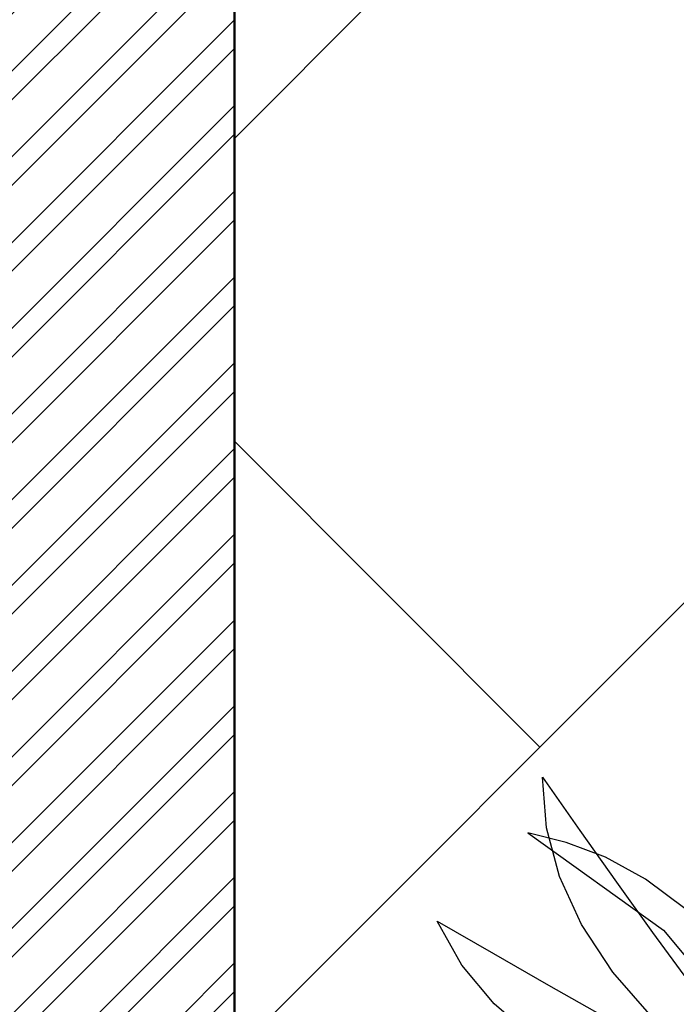
# Model space of a CAD drawing. Units: inches. Extents: x 3590 to 5167, y 65 to 1917.
# Tile 33 of 100: x 4927 to 4947, y 1357 to 1388. Entities that reach past the tile are written whole.
import ezdxf

# ---------------------------------------------------------------- set-up
doc = ezdxf.new("R2010")
doc.units = ezdxf.units.IN
for name, color, linetype, lineweight in [('A-FLOR-PATT', 8, 'Continuous', 13), ('A-WALL', 7, 'Continuous', 50), ('A-WALL-PATT', 251, 'Continuous', 13), ('L-PLNT', 94, 'Continuous', 18)]:
    doc.layers.add(name, color=color, linetype=linetype, lineweight=lineweight)
doc.layers.add('DIENHOA', color=3, linetype='Continuous')

# ---------------------------------------------------------------- blocks, each defined once
blk = doc.blocks.new('Cay03_mb')
at = {"layer": 'DIENHOA'}
for p, q in [((-365.2, 390.3), (-414.4, 402.8)), ((-414.4, 402.8), (-240.2, 277.8)), ((-314.9, 371.3), (-365.2, 390.3)), ((-263.5, 343.5), (-314.9, 371.3)), ((-211.2, 304.6), (-263.5, 343.5)), ((-240.2, 277.8), (-88.4, 94.9))]:
    blk.add_line(p, q, dxfattribs=at)
for points in [[(-395.6, 473.7), (-347.5, 405.6), (-300.6, 339.5), (-254.3, 275.1), (-208.3, 212.3), (-161.9, 150.9), (-114.8, 90.7), (-66.5, 31.6), (-16.4, -26.7)], [(-16.4, -26.7), (-108.3, 38.6), (-186.9, 101.7), (-252.4, 163.5), (-305.1, 224.4), (-345.4, 285.2), (-373.7, 346.6), (-390.4, 409.2), (-395.6, 473.7)], [(-530.5, 289.7), (-458.3, 248.1), (-387.9, 207.8), (-318.9, 168.7), (-250.8, 131.1), (-182.9, 94.8), (-114.9, 59.9), (-46.2, 26.5), (23.7, -5.4)], [(23.7, -5.4), (-87.2, 15.2), (-185, 39.6), (-270.3, 68.2), (-343.7, 101.4), (-405.9, 139.7), (-457.3, 183.5), (-498.7, 233.4), (-530.5, 289.7)]]:
    blk.add_lwpolyline(points, dxfattribs=at)

msp = doc.modelspace()

# ---------------------------------------------------------------- hatches: boundary and pattern name
at = {"layer": 'A-FLOR-PATT', "transparency": 33554687}
h = msp.add_hatch(dxfattribs=at)
h.set_pattern_fill('AR-HBONE', color=256, scale=0.2)
h.set_pattern_definition([(45, (-588.972, 0), (0, 28.73682), [60.96, -20.32]), (135, (-574.604, 14.368), (3e-15, 28.73682), [60.96, -20.32])])
h.paths.add_polyline_path([(5071.274, 1796.999), (4933.274, 1796.999), (4933.274, 1753.999), (4962.774, 1753.999, -0.414214), (4928.774, 1719.999), (4933.274, 1718.999), (4933.274, 1334.999), (5071.274, 1334.999)])
h.paths.add_polyline_path([(4951.78, 1521.077), (4951.715, 1521.04), (4951.563, 1520.895)], flags=16)
h.paths.add_polyline_path([(4952.267, 1521.376), (4952.198, 1521.371), (4952.198, 1521.356)], flags=0)
h.paths.add_polyline_path([(4967.051, 1529.728), (4965.231, 1528.694), (4963.411, 1527.714), (4961.756, 1526.851), (4963.589, 1527.449), (4964.036, 1527.478), (4962.975, 1527.249), (4961.76, 1526.852), (4959.792, 1525.834), (4958.005, 1524.895), (4956.24, 1523.93), (4954.504, 1522.919), (4954.129, 1522.682), (4953.361, 1521.997), (4953.366, 1521.998), (4953.605, 1522.064), (4955.106, 1522.761), (4956.921, 1523.434), (4958.678, 1523.915), (4960.358, 1524.2), (4961.945, 1524.286), (4964.171, 1524.108), (4965.958, 1523.309), (4963.863, 1522.976), (4965.187, 1522.499), (4963.366, 1522.497), (4961.545, 1522.487), (4959.764, 1522.461), (4958.304, 1522.419), (4957.974, 1522.388), (4956.307, 1522.232), (4954.718, 1522.071), (4953.251, 1521.899), (4953.525, 1521.623), (4954.331, 1521.379), (4956.243, 1521.23), (4958.039, 1520.93), (4959.684, 1520.483), (4961.16, 1519.896), (4963.107, 1518.8), (4964.393, 1517.325), (4962.973, 1517.726), (4964.558, 1516.661), (4965.407, 1515.708), (4963.507, 1516.322), (4961.68, 1517.005), (4959.935, 1517.745), (4958.282, 1518.528), (4956.732, 1519.343), (4955.295, 1520.175), (4954.672, 1520.572), (4954.513, 1520.627), (4955.658, 1519.318), (4956.703, 1517.982), (4957.644, 1516.647), (4958.485, 1515.334), (4959.55, 1513.524), (4960.438, 1511.769), (4958.841, 1513.62), (4957.452, 1515.325), (4955.819, 1517.459), (4956.665, 1515.448), (4957.111, 1513.923), (4957.447, 1511.714), (4957.076, 1509.793), (4956.538, 1511.11), (4955.992, 1512.569), (4955.444, 1514.125), (4954.898, 1515.735), (4954.357, 1517.356), (4953.824, 1518.943), (4953.305, 1520.452), (4953.065, 1521.116), (4952.971, 1521.146), (4952.949, 1521.086), (4952.73, 1520.199), (4953.37, 1518.024), (4953.757, 1516.373), (4954.051, 1514.765), (4954.264, 1513.221), (4954.471, 1511.131), (4954.497, 1510.402), (4954.409, 1511.76), (4954.264, 1513.221), (4954.051, 1514.765), (4953.757, 1516.373), (4953.37, 1518.024), (4952.877, 1519.698), (4952.716, 1520.141), (4952.533, 1519.059), (4952.374, 1517.789), (4952.219, 1516.312), (4952.046, 1514.6), (4951.833, 1512.626), (4951.557, 1510.363), (4951.203, 1512.168), (4950.852, 1514.339), (4950.985, 1516.376), (4951.66, 1518.286), (4952.593, 1520.481), (4952.357, 1521.13), (4951.855, 1520.328), (4950.839, 1518.908), (4949.777, 1517.587), (4948.916, 1516.617), (4948.111, 1515.256), (4947.089, 1513.554), (4945.889, 1511.615), (4946.326, 1513.402), (4946.562, 1514.249), (4945.528, 1513.327), (4944.581, 1512.531), (4946.018, 1514.508), (4947.204, 1516.048), (4947.893, 1517.313), (4949.307, 1518.764), (4950.414, 1519.767), (4950.451, 1519.806), (4952.267, 1521.376), (4951.645, 1521.493), (4950.404, 1521.18), (4948.044, 1520.359), (4946.119, 1519.452), (4944.572, 1518.475), (4943.35, 1517.443), (4941.997, 1515.92), (4941.661, 1515.275), (4942.813, 1516.99), (4944.572, 1518.475), (4946.119, 1519.452), (4948.044, 1520.359), (4950.404, 1521.18), (4951.645, 1521.493), (4949.647, 1521.868), (4948.6, 1521.756), (4947.126, 1521.57), (4945.42, 1521.348), (4943.45, 1521.105), (4941.183, 1520.856), (4942.86, 1521.613), (4943.873, 1522.03), (4942.952, 1521.909), (4941.41, 1521.485), (4939.543, 1520.67), (4938.968, 1520.226), (4940.733, 1521.299), (4942.952, 1521.909), (4943.702, 1522.008), (4945.894, 1522.7), (4947.565, 1522.714), (4948.921, 1522.566), (4951.131, 1522.183), (4950.971, 1522.297), (4948.129, 1523.006), (4946.035, 1523.707), (4944.232, 1524.521), (4942.707, 1525.461), (4941.444, 1526.537), (4940.43, 1527.761), (4939.649, 1529.143), (4941.421, 1528.122), (4943.147, 1527.132), (4944.841, 1526.175), (4946.514, 1525.25), (4948.179, 1524.359), (4948.365, 1524.263), (4946.475, 1526.045), (4945.181, 1527.54), (4944.19, 1529.033), (4943.496, 1530.54), (4943.278, 1531.36), (4942.498, 1531.919), (4943.114, 1531.762), (4942.959, 1533.659), (4944.14, 1531.989), (4944.612, 1531.323), (4946.202, 1530.463), (4947.486, 1529.509), (4948.79, 1528.226), (4950.368, 1526.237), (4949.485, 1528.155), (4948.851, 1530.123), (4948.491, 1532.041), (4948.381, 1533.918), (4948.501, 1535.76), (4948.827, 1537.573), (4949.418, 1535.565), (4949.957, 1533.569), (4950.464, 1531.586), (4950.961, 1529.617), (4951.391, 1527.954), (4951.724, 1530.687), (4952.201, 1532.58), (4952.889, 1534.33), (4953.77, 1535.951), (4954.827, 1537.46), (4954.521, 1535.39), (4954.273, 1533.937), (4955.58, 1535.663), (4956.748, 1536.739), (4956.159, 1534.78), (4955.589, 1532.873), (4955.043, 1531.006), (4954.525, 1529.166), (4954.038, 1527.341), (4953.638, 1525.733), (4953.611, 1525.586), (4953.398, 1524.166), (4953.382, 1524.009), (4954.07, 1525.476), (4954.912, 1527.022), (4956.136, 1528.894), (4957.847, 1530.577), (4959.376, 1531.54), (4958.256, 1530.104), (4957.143, 1528.663), (4956.066, 1527.243), (4955.056, 1525.871), (4954.141, 1524.571), (4953.352, 1523.372), (4953.311, 1523.303), (4953.273, 1522.925), (4953.261, 1522.382), (4954.103, 1523.373), (4954.63, 1524.284), (4955.961, 1526.358), (4957.23, 1528.13), (4958.421, 1529.609), (4960.037, 1531.368), (4961.374, 1532.375), (4962.101, 1532.77), (4961.07, 1531.061), (4959.987, 1529.438), (4958.869, 1527.908), (4958.15, 1527.007), (4959.803, 1528.003), (4961.589, 1528.793), (4963.391, 1529.328), (4965.211, 1529.632)], flags=16)
h.paths.add_polyline_path([(4962.944, 1523.182), (4961.107, 1523.422), (4960.392, 1523.362), (4962.35, 1523.331)], flags=0)
h.paths.add_polyline_path([(5049.541, 1584.551), (5049.476, 1584.515), (5049.325, 1584.37)], flags=16)
h.paths.add_polyline_path([(5050.028, 1584.851), (5049.959, 1584.845), (5049.959, 1584.83)], flags=0)
h.paths.add_polyline_path([(5042.333, 1581.949), (5043.88, 1582.926), (5045.806, 1583.833), (5048.165, 1584.654), (5049.406, 1584.967), (5047.408, 1585.342), (5046.361, 1585.231), (5044.888, 1585.044), (5043.181, 1584.822), (5041.211, 1584.579), (5038.944, 1584.33), (5040.622, 1585.087), (5041.634, 1585.504), (5040.713, 1585.383), (5039.171, 1584.959), (5037.304, 1584.144), (5036.729, 1583.7), (5038.494, 1584.773), (5040.713, 1585.383), (5041.463, 1585.482), (5043.655, 1586.174), (5045.326, 1586.188), (5046.682, 1586.04), (5048.893, 1585.657), (5048.732, 1585.771), (5045.891, 1586.48), (5043.796, 1587.181), (5041.994, 1587.996), (5040.468, 1588.935), (5039.205, 1590.011), (5038.191, 1591.235), (5037.41, 1592.617), (5039.182, 1591.596), (5040.909, 1590.607), (5042.602, 1589.649), (5044.275, 1588.724), (5045.94, 1587.833), (5046.126, 1587.738), (5044.237, 1589.519), (5042.942, 1591.015), (5041.952, 1592.508), (5041.257, 1594.014), (5041.039, 1594.834), (5040.26, 1595.393), (5040.875, 1595.237), (5040.721, 1597.133), (5041.901, 1595.463), (5042.373, 1594.798), (5043.963, 1593.938), (5045.247, 1592.983), (5046.552, 1591.701), (5048.129, 1589.712), (5047.247, 1591.63), (5046.613, 1593.597), (5046.252, 1595.515), (5046.142, 1597.392), (5046.262, 1599.234), (5046.588, 1601.047), (5047.179, 1599.039), (5047.718, 1597.043), (5048.225, 1595.06), (5048.722, 1593.091), (5049.152, 1591.429), (5049.485, 1594.161), (5049.962, 1596.054), (5050.65, 1597.804), (5051.532, 1599.425), (5052.589, 1600.934), (5052.283, 1598.864), (5052.034, 1597.411), (5053.341, 1599.137), (5054.509, 1600.213), (5053.92, 1598.254), (5053.35, 1596.348), (5052.805, 1594.48), (5052.286, 1592.64), (5051.799, 1590.815), (5051.4, 1589.207), (5051.373, 1589.06), (5051.159, 1587.64), (5051.143, 1587.483), (5051.831, 1588.95), (5052.673, 1590.496), (5053.898, 1592.368), (5055.608, 1594.051), (5057.137, 1595.014), (5056.017, 1593.578), (5054.904, 1592.137), (5053.828, 1590.717), (5052.817, 1589.345), (5051.902, 1588.046), (5051.113, 1586.846), (5051.072, 1586.777), (5051.034, 1586.399), (5051.022, 1585.856), (5051.864, 1586.847), (5052.391, 1587.758), (5053.723, 1589.832), (5054.991, 1591.604), (5056.182, 1593.083), (5057.798, 1594.842), (5059.135, 1595.849), (5059.863, 1596.244), (5058.831, 1594.535), (5057.749, 1592.912), (5056.63, 1591.382), (5055.912, 1590.482), (5057.564, 1591.477), (5059.35, 1592.267), (5061.152, 1592.802), (5062.972, 1593.106), (5064.812, 1593.203), (5062.992, 1592.169), (5061.172, 1591.188), (5059.518, 1590.325), (5061.35, 1590.924), (5061.797, 1590.952), (5060.737, 1590.723), (5059.521, 1590.326), (5057.553, 1589.308), (5055.766, 1588.369), (5054.002, 1587.404), (5052.265, 1586.393), (5051.891, 1586.156), (5051.122, 1585.471), (5051.127, 1585.472), (5051.366, 1585.538), (5052.867, 1586.235), (5054.682, 1586.908), (5056.439, 1587.389), (5058.12, 1587.675), (5059.706, 1587.76), (5061.933, 1587.583), (5063.719, 1586.783), (5061.624, 1586.45), (5062.949, 1585.973), (5061.127, 1585.971), (5059.307, 1585.961), (5057.525, 1585.935), (5056.065, 1585.893), (5055.735, 1585.862), (5054.068, 1585.707), (5052.479, 1585.546), (5051.012, 1585.373), (5051.286, 1585.097), (5052.092, 1584.853), (5054.004, 1584.704), (5055.8, 1584.404), (5057.446, 1583.958), (5058.921, 1583.37), (5060.868, 1582.274), (5062.154, 1580.799), (5060.734, 1581.2), (5062.32, 1580.135), (5063.168, 1579.182), (5061.269, 1579.796), (5059.441, 1580.479), (5057.696, 1581.219), (5056.043, 1582.003), (5054.493, 1582.817), (5053.057, 1583.649), (5052.433, 1584.047), (5052.274, 1584.101), (5053.42, 1582.793), (5054.464, 1581.457), (5055.405, 1580.121), (5056.247, 1578.809), (5057.311, 1576.998), (5058.199, 1575.244), (5056.602, 1577.094), (5055.213, 1578.799), (5053.58, 1580.933), (5054.427, 1578.922), (5054.872, 1577.397), (5055.208, 1575.189), (5054.838, 1573.267), (5054.299, 1574.584), (5053.754, 1576.043), (5053.206, 1577.599), (5052.659, 1579.209), (5052.118, 1580.83), (5051.585, 1582.417), (5051.066, 1583.927), (5050.826, 1584.59), (5050.733, 1584.62), (5050.711, 1584.561), (5050.491, 1583.673), (5051.131, 1581.498), (5051.518, 1579.847), (5051.813, 1578.24), (5052.026, 1576.695), (5052.233, 1574.605), (5052.258, 1573.876), (5052.17, 1575.234), (5052.026, 1576.695), (5051.813, 1578.24), (5051.518, 1579.847), (5051.131, 1581.498), (5050.638, 1583.172), (5050.477, 1583.615), (5050.294, 1582.533), (5050.136, 1581.263), (5049.981, 1579.786), (5049.807, 1578.074), (5049.594, 1576.1), (5049.318, 1573.837), (5048.965, 1575.642), (5048.613, 1577.813), (5048.747, 1579.85), (5049.421, 1581.76), (5050.354, 1583.955), (5050.118, 1584.604), (5049.616, 1583.802), (5048.6, 1582.382), (5047.538, 1581.061), (5046.677, 1580.091), (5045.872, 1578.73), (5044.85, 1577.028), (5043.651, 1575.089), (5044.087, 1576.877), (5044.324, 1577.723), (5043.289, 1576.801), (5042.342, 1576.005), (5043.779, 1577.982), (5044.966, 1579.522), (5045.655, 1580.787), (5047.068, 1582.239), (5048.175, 1583.241), (5048.213, 1583.28), (5050.028, 1584.851), (5049.406, 1584.967), (5048.165, 1584.654), (5045.806, 1583.833), (5043.88, 1582.926), (5042.333, 1581.949), (5041.111, 1580.917), (5039.758, 1579.394), (5039.423, 1578.749), (5040.575, 1580.464)], flags=16)
h.paths.add_polyline_path([(4954.799, 1533.12), (4954.262, 1532.079), (4953.831, 1530.935), (4953.505, 1529.636), (4953.283, 1528.133), (4953.167, 1526.376), (4953.156, 1524.315), (4953.277, 1521.236), (4952.802, 1521.842), (4951.557, 1521.998), (4950.976, 1521.961), (4952.661, 1521.941), (4952.802, 1521.842), (4953.152, 1523.593), (4953.167, 1526.376), (4953.283, 1528.133), (4953.609, 1530.346), (4954.456, 1532.592)], flags=0)
h.paths.add_polyline_path([(5050.563, 1585.316), (5049.318, 1585.472), (5048.737, 1585.435), (5050.422, 1585.415), (5050.563, 1585.316), (5050.914, 1587.067), (5050.928, 1589.851), (5051.045, 1591.607), (5051.371, 1593.82), (5052.217, 1596.066), (5052.56, 1596.594), (5052.024, 1595.554), (5051.592, 1594.409), (5051.266, 1593.11), (5051.045, 1591.607), (5050.928, 1589.851), (5050.918, 1587.789), (5051.038, 1584.71)], flags=0)
h.paths.add_polyline_path([(5058.153, 1586.836), (5060.111, 1586.805), (5060.705, 1586.656), (5058.868, 1586.896)], flags=0)
h.paths.add_polyline_path([(5049.541, 1430.936), (5049.476, 1430.9), (5049.325, 1430.755)], flags=16)
h.paths.add_polyline_path([(5050.028, 1431.236), (5049.959, 1431.231), (5049.959, 1431.215)], flags=0)
h.paths.add_polyline_path([(5046.588, 1447.432), (5047.179, 1445.425), (5047.718, 1443.429), (5048.225, 1441.446), (5048.722, 1439.476), (5049.152, 1437.814), (5049.485, 1440.546), (5049.962, 1442.439), (5050.65, 1444.189), (5051.532, 1445.811), (5052.589, 1447.319), (5052.283, 1445.249), (5052.034, 1443.796), (5053.341, 1445.522), (5054.509, 1446.598), (5053.92, 1444.64), (5053.35, 1442.733), (5052.805, 1440.865), (5052.286, 1439.025), (5051.799, 1437.201), (5051.4, 1435.592), (5051.373, 1435.445), (5051.159, 1434.025), (5051.143, 1433.868), (5051.831, 1435.335), (5052.673, 1436.881), (5053.898, 1438.753), (5055.608, 1440.436), (5057.137, 1441.4), (5056.017, 1439.963), (5054.904, 1438.522), (5053.828, 1437.102), (5052.817, 1435.73), (5051.902, 1434.431), (5051.113, 1433.231), (5051.072, 1433.162), (5051.034, 1432.784), (5051.022, 1432.242), (5051.864, 1433.232), (5052.391, 1434.143), (5053.723, 1436.217), (5054.991, 1437.989), (5056.182, 1439.468), (5057.798, 1441.227), (5059.135, 1442.235), (5059.863, 1442.629), (5058.831, 1440.921), (5057.749, 1439.298), (5056.63, 1437.767), (5055.912, 1436.867), (5057.564, 1437.863), (5059.35, 1438.652), (5061.152, 1439.187), (5062.972, 1439.491), (5064.812, 1439.588), (5062.992, 1438.554), (5061.172, 1437.573), (5059.518, 1436.71), (5061.35, 1437.309), (5061.797, 1437.337), (5060.737, 1437.108), (5059.521, 1436.711), (5057.553, 1435.693), (5055.766, 1434.754), (5054.002, 1433.789), (5052.265, 1432.778), (5051.891, 1432.541), (5051.122, 1431.856), (5051.127, 1431.857), (5051.366, 1431.923), (5052.867, 1432.62), (5054.682, 1433.293), (5056.439, 1433.775), (5058.12, 1434.06), (5059.706, 1434.145), (5061.933, 1433.968), (5063.719, 1433.168), (5061.624, 1432.835), (5062.949, 1432.358), (5061.127, 1432.357), (5059.307, 1432.346), (5057.525, 1432.32), (5056.065, 1432.278), (5055.735, 1432.248), (5054.068, 1432.092), (5052.479, 1431.931), (5051.012, 1431.759), (5051.286, 1431.482), (5052.092, 1431.238), (5054.004, 1431.089), (5055.8, 1430.789), (5057.446, 1430.343), (5058.921, 1429.755), (5060.868, 1428.66), (5062.154, 1427.185), (5060.734, 1427.585), (5062.32, 1426.52), (5063.168, 1425.567), (5061.269, 1426.181), (5059.441, 1426.865), (5057.696, 1427.604), (5056.043, 1428.388), (5054.493, 1429.202), (5053.057, 1430.034), (5052.433, 1430.432), (5052.274, 1430.487), (5053.42, 1429.178), (5054.464, 1427.842), (5055.405, 1426.506), (5056.247, 1425.194), (5057.311, 1423.383), (5058.199, 1421.629), (5056.602, 1423.479), (5055.213, 1425.184), (5053.58, 1427.318), (5054.427, 1425.307), (5054.872, 1423.782), (5055.208, 1421.574), (5054.838, 1419.652), (5054.299, 1420.97), (5053.754, 1422.428), (5053.206, 1423.984), (5052.659, 1425.595), (5052.118, 1427.215), (5051.585, 1428.802), (5051.066, 1430.312), (5050.826, 1430.975), (5050.733, 1431.005), (5050.711, 1430.946), (5050.491, 1430.058), (5051.131, 1427.883), (5051.518, 1426.232), (5051.813, 1424.625), (5052.026, 1423.081), (5052.233, 1420.991), (5052.258, 1420.261), (5052.17, 1421.619), (5052.026, 1423.081), (5051.813, 1424.625), (5051.518, 1426.232), (5051.131, 1427.883), (5050.638, 1429.558), (5050.477, 1430.001), (5050.294, 1428.918), (5050.136, 1427.648), (5049.981, 1426.171), (5049.807, 1424.459), (5049.594, 1422.485), (5049.318, 1420.222), (5048.965, 1422.028), (5048.613, 1424.199), (5048.747, 1426.235), (5049.421, 1428.146), (5050.354, 1430.34), (5050.118, 1430.989), (5049.616, 1430.187), (5048.6, 1428.768), (5047.538, 1427.446), (5046.677, 1426.477), (5045.872, 1425.116), (5044.85, 1423.413), (5043.651, 1421.474), (5044.087, 1423.262), (5044.324, 1424.109), (5043.289, 1423.186), (5042.342, 1422.391), (5043.779, 1424.368), (5044.966, 1425.907), (5045.655, 1427.173), (5047.068, 1428.624), (5048.175, 1429.627), (5048.213, 1429.666), (5050.028, 1431.236), (5049.406, 1431.353), (5048.165, 1431.039), (5045.806, 1430.218), (5043.88, 1429.311), (5042.333, 1428.334), (5041.111, 1427.302), (5039.758, 1425.779), (5039.423, 1425.134), (5040.575, 1426.849), (5042.333, 1428.334), (5043.88, 1429.311), (5045.806, 1430.218), (5048.165, 1431.039), (5049.406, 1431.353), (5047.408, 1431.727), (5046.361, 1431.616), (5044.888, 1431.429), (5043.181, 1431.207), (5041.211, 1430.964), (5038.944, 1430.715), (5040.622, 1431.472), (5041.634, 1431.89), (5040.713, 1431.769), (5039.171, 1431.345), (5037.304, 1430.53), (5036.729, 1430.085), (5038.494, 1431.158), (5040.713, 1431.769), (5041.463, 1431.867), (5043.655, 1432.559), (5045.326, 1432.573), (5046.682, 1432.425), (5048.893, 1432.042), (5048.732, 1432.156), (5045.891, 1432.865), (5043.796, 1433.566), (5041.994, 1434.381), (5040.468, 1435.321), (5039.205, 1436.396), (5038.191, 1437.62), (5037.41, 1439.002), (5039.182, 1437.982), (5040.909, 1436.992), (5042.602, 1436.034), (5044.275, 1435.109), (5045.94, 1434.218), (5046.126, 1434.123), (5044.237, 1435.904), (5042.942, 1437.4), (5041.952, 1438.893), (5041.257, 1440.399), (5041.039, 1441.219), (5040.26, 1441.778), (5040.875, 1441.622), (5040.721, 1443.518), (5041.901, 1441.848), (5042.373, 1441.183), (5043.963, 1440.323), (5045.247, 1439.369), (5046.552, 1438.086), (5048.129, 1436.097), (5047.247, 1438.015), (5046.613, 1439.982), (5046.252, 1441.901), (5046.142, 1443.778), (5046.262, 1445.619)], flags=16)
h.paths.add_polyline_path([(5052.382, 1444.255), (5051.623, 1442.78), (5052.024, 1441.939), (5052.56, 1442.98)], flags=0)
h.paths.add_polyline_path([(5050.563, 1431.701), (5049.318, 1431.857), (5048.737, 1431.821), (5050.422, 1431.8)], flags=0)
h.paths.add_polyline_path([(5058.153, 1433.221), (5060.111, 1433.19), (5060.705, 1433.041), (5058.868, 1433.281)], flags=0)
h.paths.add_polyline_path([(5049.541, 1352.285), (5049.476, 1352.249), (5049.325, 1352.104)], flags=16)
h.paths.add_polyline_path([(5050.028, 1352.585), (5049.959, 1352.58), (5049.959, 1352.564)], flags=0)
h.paths.add_polyline_path([(5046.588, 1368.781), (5047.179, 1366.774), (5047.718, 1364.778), (5048.225, 1362.795), (5048.722, 1360.825), (5049.152, 1359.163), (5049.485, 1361.896), (5049.962, 1363.789), (5050.65, 1365.538), (5051.532, 1367.16), (5052.589, 1368.669), (5052.283, 1366.598), (5052.034, 1365.145), (5053.341, 1366.871), (5054.509, 1367.947), (5053.92, 1365.989), (5053.35, 1364.082), (5052.805, 1362.214), (5052.286, 1360.374), (5051.799, 1358.55), (5051.4, 1356.942), (5051.373, 1356.794), (5051.159, 1355.374), (5051.143, 1355.218), (5051.831, 1356.684), (5052.673, 1358.23), (5053.898, 1360.102), (5055.608, 1361.786), (5057.137, 1362.749), (5056.017, 1361.313), (5054.904, 1359.872), (5053.828, 1358.452), (5052.817, 1357.079), (5051.902, 1355.78), (5051.113, 1354.581), (5051.072, 1354.512), (5051.034, 1354.133), (5051.022, 1353.591), (5051.864, 1354.581), (5052.391, 1355.492), (5053.723, 1357.566), (5054.991, 1359.338), (5056.182, 1360.817), (5057.798, 1362.577), (5059.135, 1363.584), (5059.863, 1363.979), (5058.831, 1362.27), (5057.749, 1360.647), (5056.63, 1359.117), (5055.912, 1358.216), (5057.564, 1359.212), (5059.35, 1360.001), (5061.152, 1360.536), (5062.972, 1360.841), (5064.812, 1360.937), (5062.992, 1359.903), (5061.172, 1358.923), (5059.518, 1358.059), (5061.35, 1358.658), (5061.797, 1358.687), (5060.737, 1358.458), (5059.521, 1358.061), (5057.553, 1357.043), (5055.766, 1356.103), (5054.002, 1355.138), (5052.265, 1354.127), (5051.891, 1353.89), (5051.122, 1353.206), (5051.127, 1353.206), (5051.366, 1353.272), (5052.867, 1353.969), (5054.682, 1354.643), (5056.439, 1355.124), (5058.12, 1355.409), (5059.706, 1355.495), (5061.933, 1355.317), (5063.719, 1354.518), (5061.624, 1354.184), (5062.949, 1353.708), (5061.127, 1353.706), (5059.307, 1353.695), (5057.525, 1353.669), (5056.065, 1353.627), (5055.735, 1353.597), (5054.068, 1353.441), (5052.479, 1353.28), (5051.012, 1353.108), (5051.286, 1352.831), (5052.092, 1352.587), (5054.004, 1352.439), (5055.8, 1352.138), (5057.446, 1351.692), (5058.921, 1351.104), (5060.868, 1350.009), (5062.154, 1348.534), (5060.734, 1348.935), (5062.32, 1347.869), (5063.168, 1346.916), (5061.269, 1347.53), (5059.441, 1348.214), (5057.696, 1348.954), (5056.043, 1349.737), (5054.493, 1350.551), (5053.057, 1351.383), (5052.433, 1351.781), (5052.274, 1351.836), (5053.42, 1350.527), (5054.464, 1349.191), (5055.405, 1347.855), (5056.247, 1346.543), (5057.311, 1344.733), (5058.199, 1342.978), (5056.602, 1344.828), (5055.213, 1346.534), (5053.58, 1348.667), (5054.427, 1346.656), (5054.872, 1345.132), (5055.208, 1342.923), (5054.838, 1341.002), (5054.299, 1342.319), (5053.754, 1343.778), (5053.206, 1345.334), (5052.659, 1346.944), (5052.118, 1348.564), (5051.585, 1350.151), (5051.066, 1351.661), (5050.826, 1352.324), (5050.733, 1352.355), (5050.711, 1352.295), (5050.491, 1351.408), (5051.131, 1349.232), (5051.518, 1347.581), (5051.813, 1345.974), (5052.026, 1344.43), (5052.233, 1342.34), (5052.258, 1341.61), (5052.17, 1342.969), (5052.026, 1344.43), (5051.813, 1345.974), (5051.518, 1347.581), (5051.131, 1349.232), (5050.638, 1350.907), (5050.477, 1351.35), (5050.294, 1350.267), (5050.136, 1348.997), (5049.981, 1347.52), (5049.807, 1345.809), (5049.594, 1343.835), (5049.318, 1341.571), (5048.965, 1343.377), (5048.613, 1345.548), (5048.747, 1347.585), (5049.421, 1349.495), (5050.354, 1351.689), (5050.118, 1352.339), (5049.616, 1351.536), (5048.6, 1350.117), (5047.538, 1348.795), (5046.677, 1347.826), (5045.872, 1346.465), (5044.85, 1344.763), (5043.651, 1342.824), (5044.087, 1344.611), (5044.324, 1345.458), (5043.289, 1344.535), (5042.342, 1343.74), (5043.779, 1345.717), (5044.966, 1347.256), (5045.655, 1348.522), (5047.068, 1349.973), (5048.175, 1350.976), (5048.213, 1351.015), (5050.028, 1352.585), (5049.406, 1352.702), (5048.165, 1352.388), (5045.806, 1351.567), (5043.88, 1350.661), (5042.333, 1349.683), (5041.111, 1348.651), (5039.758, 1347.128), (5039.423, 1346.483), (5040.575, 1348.198), (5042.333, 1349.683), (5043.88, 1350.661), (5045.806, 1351.567), (5048.165, 1352.388), (5049.406, 1352.702), (5047.408, 1353.076), (5046.361, 1352.965), (5044.888, 1352.779), (5043.181, 1352.556), (5041.211, 1352.313), (5038.944, 1352.065), (5040.622, 1352.821), (5041.634, 1353.239), (5040.713, 1353.118), (5039.171, 1352.694), (5037.304, 1351.879), (5036.729, 1351.434), (5038.494, 1352.508), (5040.713, 1353.118), (5041.463, 1353.216), (5043.655, 1353.909), (5045.326, 1353.923), (5046.682, 1353.774), (5048.893, 1353.391), (5048.732, 1353.506), (5045.891, 1354.214), (5043.796, 1354.915), (5041.994, 1355.73), (5040.468, 1356.67), (5039.205, 1357.746), (5038.191, 1358.969), (5037.41, 1360.352), (5039.182, 1359.331), (5040.909, 1358.341), (5042.602, 1357.383), (5044.275, 1356.458), (5045.94, 1355.567), (5046.126, 1355.472), (5044.237, 1357.253), (5042.942, 1358.749), (5041.952, 1360.242), (5041.257, 1361.748), (5041.039, 1362.568), (5040.26, 1363.128), (5040.875, 1362.971), (5040.721, 1364.867), (5041.901, 1363.197), (5042.373, 1362.532), (5043.963, 1361.672), (5045.247, 1360.718), (5046.552, 1359.435), (5048.129, 1357.446), (5047.247, 1359.364), (5046.613, 1361.331), (5046.252, 1363.25), (5046.142, 1365.127), (5046.262, 1366.969)], flags=16)
h.paths.add_polyline_path([(5052.382, 1365.604), (5051.623, 1364.129), (5052.024, 1363.288), (5052.56, 1364.329)], flags=0)
h.paths.add_polyline_path([(4951.78, 1698.041), (4951.715, 1698.005), (4951.563, 1697.859)], flags=16)
h.paths.add_polyline_path([(4952.267, 1698.341), (4952.198, 1698.335), (4952.198, 1698.32)], flags=0)
h.paths.add_polyline_path([(4957.076, 1686.757), (4956.538, 1688.074), (4955.992, 1689.533), (4955.444, 1691.089), (4954.898, 1692.699), (4954.357, 1694.32), (4953.824, 1695.907), (4953.305, 1697.417), (4953.065, 1698.08), (4952.971, 1698.11), (4952.949, 1698.051), (4952.73, 1697.163), (4953.37, 1694.988), (4953.757, 1693.337), (4954.051, 1691.729), (4954.264, 1690.185), (4954.471, 1688.095), (4954.497, 1687.366), (4954.409, 1688.724), (4954.264, 1690.185), (4954.051, 1691.729), (4953.757, 1693.337), (4953.37, 1694.988), (4952.877, 1696.662), (4952.716, 1697.105), (4952.533, 1696.023), (4952.374, 1694.753), (4952.219, 1693.276), (4952.046, 1691.564), (4951.833, 1689.59), (4951.557, 1687.327), (4951.203, 1689.132), (4950.852, 1691.303), (4950.985, 1693.34), (4951.66, 1695.25), (4952.593, 1697.445), (4952.357, 1698.094), (4951.855, 1697.292), (4950.839, 1695.872), (4949.777, 1694.551), (4948.916, 1693.581), (4948.111, 1692.22), (4947.089, 1690.518), (4945.889, 1688.579), (4946.326, 1690.366), (4946.562, 1691.213), (4945.528, 1690.291), (4944.581, 1689.495), (4946.018, 1691.472), (4947.204, 1693.012), (4947.893, 1694.277), (4949.307, 1695.729), (4950.414, 1696.731), (4950.451, 1696.77), (4952.267, 1698.341), (4951.645, 1698.457), (4950.404, 1698.144), (4948.044, 1697.323), (4946.119, 1696.416), (4944.572, 1695.439), (4943.35, 1694.407), (4941.997, 1692.884), (4941.661, 1692.239), (4942.813, 1693.954), (4944.572, 1695.439), (4946.119, 1696.416), (4948.044, 1697.323), (4950.404, 1698.144), (4951.645, 1698.457), (4949.647, 1698.832), (4948.6, 1698.72), (4947.126, 1698.534), (4945.42, 1698.312), (4943.45, 1698.069), (4941.183, 1697.82), (4942.86, 1698.577), (4943.873, 1698.994), (4942.952, 1698.873), (4941.41, 1698.449), (4939.543, 1697.634), (4938.968, 1697.19), (4940.733, 1698.263), (4942.952, 1698.873), (4943.702, 1698.972), (4945.894, 1699.664), (4947.565, 1699.678), (4948.921, 1699.53), (4951.131, 1699.147), (4950.971, 1699.261), (4948.129, 1699.97), (4946.035, 1700.671), (4944.232, 1701.486), (4942.707, 1702.425), (4941.444, 1703.501), (4940.43, 1704.725), (4939.649, 1706.107), (4941.421, 1705.086), (4943.147, 1704.097), (4944.841, 1703.139), (4946.514, 1702.214), (4948.179, 1701.323), (4948.365, 1701.227), (4946.475, 1703.009), (4945.181, 1704.505), (4944.19, 1705.997), (4943.496, 1707.504), (4943.278, 1708.324), (4942.498, 1708.883), (4943.114, 1708.727), (4942.959, 1710.623), (4944.14, 1708.953), (4944.612, 1708.287), (4946.202, 1707.428), (4947.486, 1706.473), (4948.79, 1705.191), (4950.368, 1703.202), (4949.485, 1705.12), (4948.851, 1707.087), (4948.491, 1709.005), (4948.381, 1710.882), (4948.501, 1712.724), (4948.827, 1714.537), (4949.418, 1712.529), (4949.957, 1710.533), (4950.464, 1708.55), (4950.961, 1706.581), (4951.391, 1704.919), (4951.724, 1707.651), (4952.201, 1709.544), (4952.889, 1711.294), (4953.77, 1712.915), (4954.827, 1714.424), (4954.521, 1712.354), (4954.273, 1710.901), (4955.58, 1712.627), (4956.748, 1713.703), (4956.159, 1711.744), (4955.589, 1709.837), (4955.043, 1707.97), (4954.525, 1706.13), (4954.038, 1704.305), (4953.638, 1702.697), (4953.611, 1702.55), (4953.398, 1701.13), (4953.382, 1700.973), (4954.07, 1702.44), (4954.912, 1703.986), (4956.136, 1705.858), (4957.847, 1707.541), (4959.376, 1708.504), (4958.256, 1707.068), (4957.143, 1705.627), (4956.066, 1704.207), (4955.056, 1702.835), (4954.141, 1701.536), (4953.352, 1700.336), (4953.311, 1700.267), (4953.273, 1699.889), (4953.261, 1699.346), (4954.103, 1700.337), (4954.63, 1701.248), (4955.961, 1703.322), (4957.23, 1705.094), (4958.421, 1706.573), (4960.037, 1708.332), (4961.374, 1709.339), (4962.101, 1709.734), (4961.07, 1708.025), (4959.987, 1706.402), (4958.869, 1704.872), (4958.15, 1703.972), (4959.803, 1704.967), (4961.589, 1705.757), (4963.391, 1706.292), (4965.211, 1706.596), (4967.051, 1706.692), (4965.231, 1705.659), (4963.411, 1704.678), (4961.756, 1703.815), (4963.589, 1704.413), (4964.036, 1704.442), (4962.975, 1704.213), (4961.76, 1703.816), (4959.792, 1702.798), (4958.005, 1701.859), (4956.24, 1700.894), (4954.504, 1699.883), (4954.129, 1699.646), (4953.361, 1698.961), (4953.366, 1698.962), (4953.605, 1699.028), (4955.106, 1699.725), (4956.921, 1700.398), (4958.678, 1700.879), (4960.358, 1701.164), (4961.945, 1701.25), (4964.171, 1701.073), (4965.958, 1700.273), (4963.863, 1699.94), (4965.187, 1699.463), (4963.366, 1699.461), (4961.545, 1699.451), (4959.764, 1699.425), (4958.304, 1699.383), (4957.974, 1699.352), (4956.307, 1699.197), (4954.718, 1699.036), (4953.251, 1698.863), (4953.525, 1698.587), (4954.331, 1698.343), (4956.243, 1698.194), (4958.039, 1697.894), (4959.684, 1697.447), (4961.16, 1696.86), (4963.107, 1695.764), (4964.393, 1694.289), (4962.973, 1694.69), (4964.558, 1693.625), (4965.407, 1692.672), (4963.507, 1693.286), (4961.68, 1693.969), (4959.935, 1694.709), (4958.282, 1695.492), (4956.732, 1696.307), (4955.295, 1697.139), (4954.672, 1697.536), (4954.513, 1697.591), (4955.658, 1696.282), (4956.703, 1694.946), (4957.644, 1693.611), (4958.485, 1692.298), (4959.55, 1690.488), (4960.438, 1688.733), (4958.841, 1690.584), (4957.452, 1692.289), (4955.819, 1694.423), (4956.665, 1692.412), (4957.111, 1690.887), (4957.447, 1688.678)], flags=16)
h.paths.add_polyline_path([(5050.563, 1353.05), (5049.318, 1353.207), (5048.737, 1353.17), (5050.422, 1353.15)], flags=0)
h.paths.add_polyline_path([(4951.78, 1351.486), (4951.715, 1351.45), (4951.563, 1351.305)], flags=16)
h.paths.add_polyline_path([(4952.267, 1351.786), (4952.198, 1351.78), (4952.198, 1351.765)], flags=0)
h.paths.add_polyline_path([(4954.827, 1367.869), (4954.521, 1365.799), (4954.273, 1364.346), (4955.58, 1366.072), (4956.748, 1367.148), (4956.159, 1365.19), (4955.589, 1363.283), (4955.043, 1361.415), (4954.525, 1359.575), (4954.038, 1357.751), (4953.638, 1356.142), (4953.611, 1355.995), (4953.398, 1354.575), (4953.382, 1354.418), (4954.07, 1355.885), (4954.912, 1357.431), (4956.136, 1359.303), (4957.847, 1360.986), (4959.376, 1361.95), (4958.256, 1360.513), (4957.143, 1359.072), (4956.066, 1357.652), (4955.056, 1356.28), (4954.141, 1354.981), (4953.352, 1353.781), (4953.311, 1353.712), (4953.273, 1353.334), (4953.261, 1352.792), (4954.103, 1353.782), (4954.63, 1354.693), (4955.961, 1356.767), (4957.23, 1358.539), (4958.421, 1360.018), (4960.037, 1361.777), (4961.374, 1362.785), (4962.101, 1363.179), (4961.07, 1361.471), (4959.987, 1359.848), (4958.869, 1358.317), (4958.15, 1357.417), (4959.803, 1358.413), (4961.589, 1359.202), (4963.391, 1359.737), (4965.211, 1360.041), (4967.051, 1360.138), (4965.231, 1359.104), (4963.411, 1358.123), (4961.756, 1357.26), (4963.589, 1357.859), (4964.036, 1357.887), (4962.975, 1357.658), (4961.76, 1357.261), (4959.792, 1356.243), (4958.005, 1355.304), (4956.24, 1354.339), (4954.504, 1353.328), (4954.129, 1353.091), (4953.361, 1352.406), (4953.366, 1352.407), (4953.605, 1352.473), (4955.106, 1353.17), (4956.921, 1353.843), (4958.678, 1354.325), (4960.358, 1354.61), (4961.945, 1354.695), (4964.171, 1354.518), (4965.958, 1353.718), (4963.863, 1353.385), (4965.187, 1352.908), (4963.366, 1352.907), (4961.545, 1352.896), (4959.764, 1352.87), (4958.304, 1352.828), (4957.974, 1352.798), (4956.307, 1352.642), (4954.718, 1352.481), (4953.251, 1352.309), (4953.525, 1352.032), (4954.331, 1351.788), (4956.243, 1351.639), (4958.039, 1351.339), (4959.684, 1350.893), (4961.16, 1350.305), (4963.107, 1349.21), (4964.393, 1347.735), (4962.973, 1348.135), (4964.558, 1347.07), (4965.407, 1346.117), (4963.507, 1346.731), (4961.68, 1347.414), (4959.935, 1348.154), (4958.282, 1348.938), (4956.732, 1349.752), (4955.295, 1350.584), (4954.672, 1350.982), (4954.513, 1351.036), (4955.658, 1349.728), (4956.703, 1348.392), (4957.644, 1347.056), (4958.485, 1345.744), (4959.55, 1343.933), (4960.438, 1342.179), (4958.841, 1344.029), (4957.452, 1345.734), (4955.819, 1347.868), (4956.665, 1345.857), (4957.111, 1344.332), (4957.447, 1342.124), (4957.076, 1340.202), (4956.538, 1341.52), (4955.992, 1342.978), (4955.444, 1344.534), (4954.898, 1346.145), (4954.357, 1347.765), (4953.824, 1349.352), (4953.305, 1350.862), (4953.065, 1351.525), (4952.971, 1351.555), (4952.949, 1351.496), (4952.73, 1350.608), (4953.37, 1348.433), (4953.757, 1346.782), (4954.051, 1345.175), (4954.264, 1343.631), (4954.471, 1341.541), (4954.497, 1340.811), (4954.409, 1342.169), (4954.264, 1343.631), (4954.051, 1345.175), (4953.757, 1346.782), (4953.37, 1348.433), (4952.877, 1350.108), (4952.716, 1350.551), (4952.533, 1349.468), (4952.374, 1348.198), (4952.219, 1346.721), (4952.046, 1345.009), (4951.833, 1343.035), (4951.557, 1340.772), (4951.203, 1342.578), (4950.852, 1344.749), (4950.985, 1346.785), (4951.66, 1348.696), (4952.593, 1350.89), (4952.357, 1351.539), (4951.855, 1350.737), (4950.839, 1349.318), (4949.777, 1347.996), (4948.916, 1347.027), (4948.111, 1345.665), (4947.089, 1343.963), (4945.889, 1342.024), (4946.326, 1343.812), (4946.562, 1344.659), (4945.528, 1343.736), (4944.581, 1342.941), (4946.018, 1344.918), (4947.204, 1346.457), (4947.893, 1347.723), (4949.307, 1349.174), (4950.414, 1350.177), (4950.451, 1350.216), (4952.267, 1351.786), (4951.645, 1351.903), (4950.404, 1351.589), (4948.044, 1350.768), (4946.119, 1349.861), (4944.572, 1348.884), (4943.35, 1347.852), (4941.997, 1346.329), (4941.661, 1345.684), (4942.813, 1347.399), (4944.572, 1348.884), (4946.119, 1349.861), (4948.044, 1350.768), (4950.404, 1351.589), (4951.645, 1351.903), (4949.647, 1352.277), (4948.6, 1352.166), (4947.126, 1351.979), (4945.42, 1351.757), (4943.45, 1351.514), (4941.183, 1351.265), (4942.86, 1352.022), (4943.873, 1352.44), (4942.952, 1352.319), (4941.41, 1351.895), (4939.543, 1351.08), (4938.968, 1350.635), (4940.733, 1351.708), (4942.952, 1352.319), (4943.702, 1352.417), (4945.894, 1353.109), (4947.565, 1353.123), (4948.921, 1352.975), (4951.131, 1352.592), (4950.971, 1352.706), (4948.129, 1353.415), (4946.035, 1354.116), (4944.232, 1354.931), (4942.707, 1355.871), (4941.444, 1356.946), (4940.43, 1358.17), (4939.649, 1359.552), (4941.421, 1358.532), (4943.147, 1357.542), (4944.841, 1356.584), (4946.514, 1355.659), (4948.179, 1354.768), (4948.365, 1354.673), (4946.475, 1356.454), (4945.181, 1357.95), (4944.19, 1359.443), (4943.496, 1360.949), (4943.278, 1361.769), (4942.498, 1362.328), (4943.114, 1362.172), (4942.959, 1364.068), (4944.14, 1362.398), (4944.612, 1361.733), (4946.202, 1360.873), (4947.486, 1359.919), (4948.79, 1358.636), (4950.368, 1356.647), (4949.485, 1358.565), (4948.851, 1360.532), (4948.491, 1362.451), (4948.381, 1364.328), (4948.501, 1366.169), (4948.827, 1367.982), (4949.418, 1365.975), (4949.957, 1363.979), (4950.464, 1361.995), (4950.961, 1360.026), (4951.391, 1358.364), (4951.724, 1361.096), (4952.201, 1362.989), (4952.889, 1364.739), (4953.77, 1366.361)], flags=16)
h.paths.add_polyline_path([(4954.799, 1363.53), (4954.262, 1362.489), (4953.831, 1361.344), (4953.505, 1360.045), (4953.283, 1358.543), (4953.167, 1356.786), (4953.156, 1354.724), (4953.277, 1351.646), (4952.802, 1352.251), (4951.557, 1352.407), (4950.976, 1352.371), (4952.661, 1352.35), (4952.802, 1352.251), (4953.152, 1354.002), (4953.167, 1356.786), (4953.283, 1358.543), (4953.609, 1360.755), (4954.456, 1363.001)], flags=0)
h.paths.add_polyline_path([(4952.802, 1698.806), (4951.557, 1698.962), (4950.976, 1698.925), (4952.661, 1698.905), (4952.802, 1698.806), (4953.152, 1700.557), (4953.167, 1703.34), (4953.283, 1705.097), (4953.609, 1707.31), (4954.456, 1709.556), (4954.799, 1710.084), (4954.262, 1709.043), (4953.831, 1707.899), (4953.505, 1706.6), (4953.283, 1705.097), (4953.167, 1703.34), (4953.156, 1701.279), (4953.277, 1698.2)], flags=0)
h.paths.add_polyline_path([(4962.944, 1700.146), (4961.107, 1700.386), (4960.392, 1700.326), (4962.35, 1700.295)], flags=0)
h.paths.add_polyline_path([(5058.153, 1354.57), (5060.111, 1354.539), (5060.705, 1354.391), (5058.868, 1354.631)], flags=0)
h.paths.add_polyline_path([(4962.944, 1353.591), (4961.107, 1353.831), (4960.392, 1353.771), (4962.35, 1353.74)], flags=0)
h.paths.add_polyline_path([(5049.541, 1778.72), (5049.476, 1778.684), (5049.325, 1778.539)], flags=16)
h.paths.add_polyline_path([(5050.028, 1779.02), (5049.959, 1779.014), (5049.959, 1778.999)], flags=0)
h.paths.add_polyline_path([(5052.258, 1768.045), (5052.17, 1769.403), (5052.026, 1770.864), (5051.813, 1772.409), (5051.518, 1774.016), (5051.131, 1775.667), (5050.638, 1777.341), (5050.477, 1777.784), (5050.294, 1776.702), (5050.136, 1775.432), (5049.981, 1773.955), (5049.807, 1772.243), (5049.594, 1770.269), (5049.318, 1768.006), (5048.965, 1769.811), (5048.613, 1771.982), (5048.747, 1774.019), (5049.421, 1775.929), (5050.354, 1778.124), (5050.118, 1778.773), (5049.616, 1777.971), (5048.6, 1776.551), (5047.538, 1775.23), (5046.677, 1774.26), (5045.872, 1772.899), (5044.85, 1771.197), (5043.651, 1769.258), (5044.087, 1771.046), (5044.324, 1771.892), (5043.289, 1770.97), (5042.342, 1770.174), (5043.779, 1772.151), (5044.966, 1773.691), (5045.655, 1774.956), (5047.068, 1776.408), (5048.175, 1777.41), (5048.213, 1777.449), (5050.028, 1779.02), (5049.406, 1779.136), (5048.165, 1778.823), (5045.806, 1778.002), (5043.88, 1777.095), (5042.333, 1776.118), (5041.111, 1775.086), (5039.758, 1773.563), (5039.423, 1772.918), (5040.575, 1774.633), (5042.333, 1776.118), (5043.88, 1777.095), (5045.806, 1778.002), (5048.165, 1778.823), (5049.406, 1779.136), (5047.408, 1779.511), (5046.361, 1779.4), (5044.888, 1779.213), (5043.181, 1778.991), (5041.211, 1778.748), (5038.944, 1778.499), (5040.622, 1779.256), (5041.634, 1779.673), (5040.713, 1779.552), (5039.171, 1779.128), (5037.304, 1778.313), (5036.729, 1777.869), (5038.494, 1778.942), (5040.713, 1779.552), (5041.463, 1779.651), (5043.655, 1780.343), (5045.326, 1780.357), (5046.682, 1780.209), (5048.893, 1779.826), (5048.732, 1779.94), (5045.891, 1780.649), (5043.796, 1781.35), (5041.994, 1782.165), (5040.468, 1783.104), (5039.205, 1784.18), (5038.191, 1785.404), (5037.41, 1786.786), (5039.182, 1785.765), (5040.909, 1784.776), (5042.602, 1783.818), (5044.275, 1782.893), (5045.94, 1782.002), (5046.126, 1781.907), (5044.237, 1783.688), (5042.942, 1785.184), (5041.952, 1786.677), (5041.257, 1788.183), (5041.039, 1789.003), (5040.26, 1789.562), (5040.875, 1789.406), (5040.721, 1791.302), (5041.901, 1789.632), (5042.373, 1788.967), (5043.963, 1788.107), (5045.247, 1787.152), (5046.552, 1785.87), (5048.129, 1783.881), (5047.247, 1785.799), (5046.613, 1787.766), (5046.252, 1789.684), (5046.142, 1791.561), (5046.262, 1793.403), (5046.588, 1795.216), (5047.179, 1793.208), (5047.718, 1791.213), (5048.225, 1789.229), (5048.722, 1787.26), (5049.152, 1785.598), (5049.485, 1788.33), (5049.962, 1790.223), (5050.65, 1791.973), (5051.532, 1793.594), (5052.589, 1795.103), (5052.283, 1793.033), (5052.034, 1791.58), (5053.341, 1793.306), (5054.509, 1794.382), (5053.92, 1792.423), (5053.35, 1790.517), (5052.805, 1788.649), (5052.286, 1786.809), (5051.799, 1784.984), (5051.4, 1783.376), (5051.373, 1783.229), (5051.159, 1781.809), (5051.143, 1781.652), (5051.831, 1783.119), (5052.673, 1784.665), (5053.898, 1786.537), (5055.608, 1788.22), (5057.137, 1789.183), (5056.017, 1787.747), (5054.904, 1786.306), (5053.828, 1784.886), (5052.817, 1783.514), (5051.902, 1782.215), (5051.113, 1781.015), (5051.072, 1780.946), (5051.034, 1780.568), (5051.022, 1780.025), (5051.864, 1781.016), (5052.391, 1781.927), (5053.723, 1784.001), (5054.991, 1785.773), (5056.182, 1787.252), (5057.798, 1789.011), (5059.135, 1790.018), (5059.863, 1790.413), (5058.831, 1788.704), (5057.749, 1787.081), (5056.63, 1785.551), (5055.912, 1784.651), (5057.564, 1785.646), (5059.35, 1786.436), (5061.152, 1786.971), (5062.972, 1787.275), (5064.812, 1787.372), (5062.992, 1786.338), (5061.172, 1785.357), (5059.518, 1784.494), (5061.35, 1785.093), (5061.797, 1785.121), (5060.737, 1784.892), (5059.521, 1784.495), (5057.553, 1783.477), (5055.766, 1782.538), (5054.002, 1781.573), (5052.265, 1780.562), (5051.891, 1780.325), (5051.122, 1779.64), (5051.127, 1779.641), (5051.366, 1779.707), (5052.867, 1780.404), (5054.682, 1781.077), (5056.439, 1781.558), (5058.12, 1781.844), (5059.706, 1781.929), (5061.933, 1781.752), (5063.719, 1780.952), (5061.624, 1780.619), (5062.949, 1780.142), (5061.127, 1780.14), (5059.307, 1780.13), (5057.525, 1780.104), (5056.065, 1780.062), (5055.735, 1780.031), (5054.068, 1779.876), (5052.479, 1779.715), (5051.012, 1779.542), (5051.286, 1779.266), (5052.092, 1779.022), (5054.004, 1778.873), (5055.8, 1778.573), (5057.446, 1778.127), (5058.921, 1777.539), (5060.868, 1776.443), (5062.154, 1774.968), (5060.734, 1775.369), (5062.32, 1774.304), (5063.168, 1773.351), (5061.269, 1773.965), (5059.441, 1774.648), (5057.696, 1775.388), (5056.043, 1776.172), (5054.493, 1776.986), (5053.057, 1777.818), (5052.433, 1778.216), (5052.274, 1778.27), (5053.42, 1776.962), (5054.464, 1775.626), (5055.405, 1774.29), (5056.247, 1772.978), (5057.311, 1771.167), (5058.199, 1769.413), (5056.602, 1771.263), (5055.213, 1772.968), (5053.58, 1775.102), (5054.427, 1773.091), (5054.872, 1771.566), (5055.208, 1769.358), (5054.838, 1767.436), (5054.299, 1768.753), (5053.754, 1770.212), (5053.206, 1771.768), (5052.659, 1773.378), (5052.118, 1774.999), (5051.585, 1776.586), (5051.066, 1778.096), (5050.826, 1778.759), (5050.733, 1778.789), (5050.711, 1778.73), (5050.491, 1777.842), (5051.131, 1775.667), (5051.518, 1774.016), (5051.813, 1772.409), (5052.026, 1770.864), (5052.233, 1768.774)], flags=16)
h.paths.add_polyline_path([(5050.563, 1779.485), (5049.318, 1779.641), (5048.737, 1779.604), (5050.422, 1779.584), (5050.563, 1779.485), (5050.914, 1781.236), (5050.928, 1784.02), (5051.045, 1785.776), (5051.371, 1787.989), (5052.217, 1790.235), (5052.56, 1790.763), (5052.024, 1789.723), (5051.592, 1788.578), (5051.266, 1787.279), (5051.045, 1785.776), (5050.928, 1784.02), (5050.918, 1781.958), (5051.038, 1778.879)], flags=0)
h.paths.add_polyline_path([(5058.153, 1781.005), (5060.111, 1780.974), (5060.705, 1780.825), (5058.868, 1781.065)], flags=0)
at = {"layer": 'A-WALL-PATT', "transparency": 33554687}
h = msp.add_hatch(dxfattribs=at)
h.set_pattern_fill('ANSI32', color=256, scale=0.2)
h.paths.add_polyline_path([(4684.274, 1805.999), (4591.274, 1805.999), (4591.274, 1796.999), (4639.274, 1796.999), (4639.274, 1790.999), (4648.274, 1790.999), (4648.274, 1796.999), (4684.274, 1796.999)])
h.paths.add_polyline_path([(4543.274, 1805.999), (4420.274, 1805.999), (4420.274, 1784.999), (4429.274, 1784.999), (4429.274, 1796.999), (4445.919, 1796.999), (4543.274, 1796.999)])
h.paths.add_polyline_path([(4828.274, 1805.999), (4744.274, 1805.999), (4744.274, 1796.999), (4828.274, 1796.999)])
h.paths.add_polyline_path([(4648.274, 1754.999), (4639.274, 1754.999), (4639.274, 1655.999), (4546.274, 1655.999), (4546.274, 1649.999), (4549.274, 1649.999), (4549.274, 1553.999), (4429.274, 1553.999), (4429.274, 1583.999), (4420.274, 1583.999), (4420.274, 1538.999), (4429.274, 1538.999), (4429.274, 1544.999), (4639.274, 1544.999), (4639.274, 1538.999), (4648.274, 1538.999), (4648.274, 1559.999), (4639.274, 1559.999), (4639.274, 1553.999), (4555.274, 1553.999), (4555.274, 1649.999), (4639.274, 1649.999), (4639.274, 1589.999), (4648.274, 1589.999)])
h.paths.add_polyline_path([(4516.274, 1655.999), (4429.274, 1655.999), (4429.274, 1736.999), (4420.274, 1736.999), (4420.274, 1619.999), (4429.274, 1619.999), (4429.274, 1649.999), (4516.274, 1649.999)], flags=17)
h.paths.add_polyline_path([(5080.274, 1805.999), (4888.274, 1805.999), (4888.274, 1796.999), (4924.274, 1796.999), (4924.274, 1754.999), (4933.274, 1754.999), (4933.274, 1796.999), (5071.274, 1796.999), (5071.274, 1334.999), (4933.274, 1334.999), (4933.274, 1565.999), (4924.274, 1565.999), (4924.274, 1334.999), (4898.774, 1334.999), (4898.774, 1325.999), (5080.274, 1325.999)])
h.paths.add_polyline_path([(4933.274, 1718.999), (4924.274, 1718.999), (4924.274, 1637.999), (4933.274, 1637.999)], flags=17)
h.paths.add_polyline_path([(4802.774, 1334.999), (4777.274, 1334.999), (4777.274, 1502.999), (4756.274, 1502.999), (4756.274, 1493.999), (4768.274, 1493.999), (4768.274, 1430.999), (4696.274, 1430.999), (4696.274, 1493.999), (4708.274, 1493.999), (4708.274, 1502.999), (4639.274, 1502.999), (4639.274, 1493.999), (4687.274, 1493.999), (4687.274, 1430.999), (4681.274, 1430.999), (4681.274, 1421.999), (4768.274, 1421.999), (4768.274, 1334.999), (4726.274, 1334.999), (4726.274, 1325.999), (4802.774, 1325.999)])
h.paths.add_polyline_path([(4690.274, 1334.999), (4648.274, 1334.999), (4648.274, 1352.867), (4648.274, 1421.999), (4651.274, 1421.999), (4651.274, 1430.999), (4639.274, 1430.999), (4639.274, 1334.999), (4633.274, 1334.999), (4633.274, 1325.999), (4690.274, 1325.999)])
h.paths.add_polyline_path([(4585.274, 1334.999), (4584.724, 1334.999), (4429.274, 1334.999), (4429.274, 1490.999), (4420.274, 1490.999), (4420.274, 1325.999), (4585.274, 1325.999)])

# ---------------------------------------------------------------- linework, layer by layer
at = {"layer": 'A-WALL'}
msp.add_line((4933.274, 1334.999), (4933.274, 1718.999), dxfattribs=at)

# ---------------------------------------------------------------- block references
at = {"layer": 'L-PLNT', "xscale": 0.0245452446402784, "yscale": 0.0245452446402784, "zscale": 0.0245452446402784}
msp.add_blockref('Cay03_mb', (4952.669, 1352.442), dxfattribs=at)

doc.saveas('drawing.dxf')
